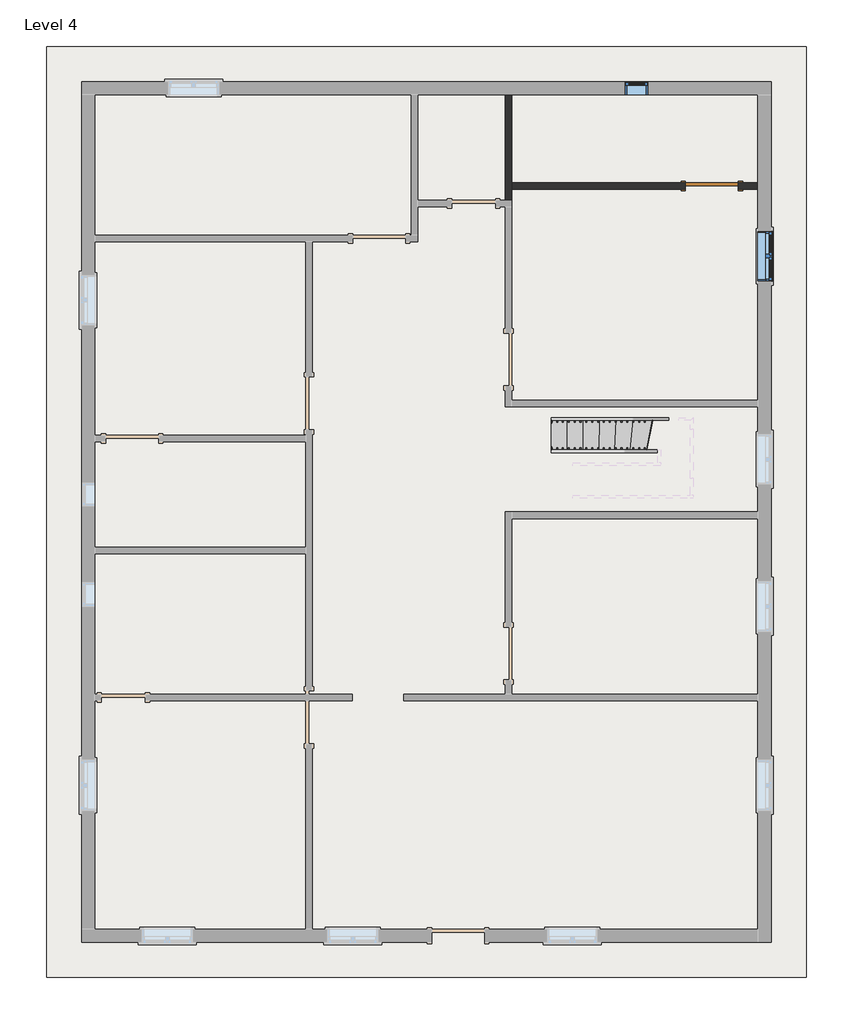
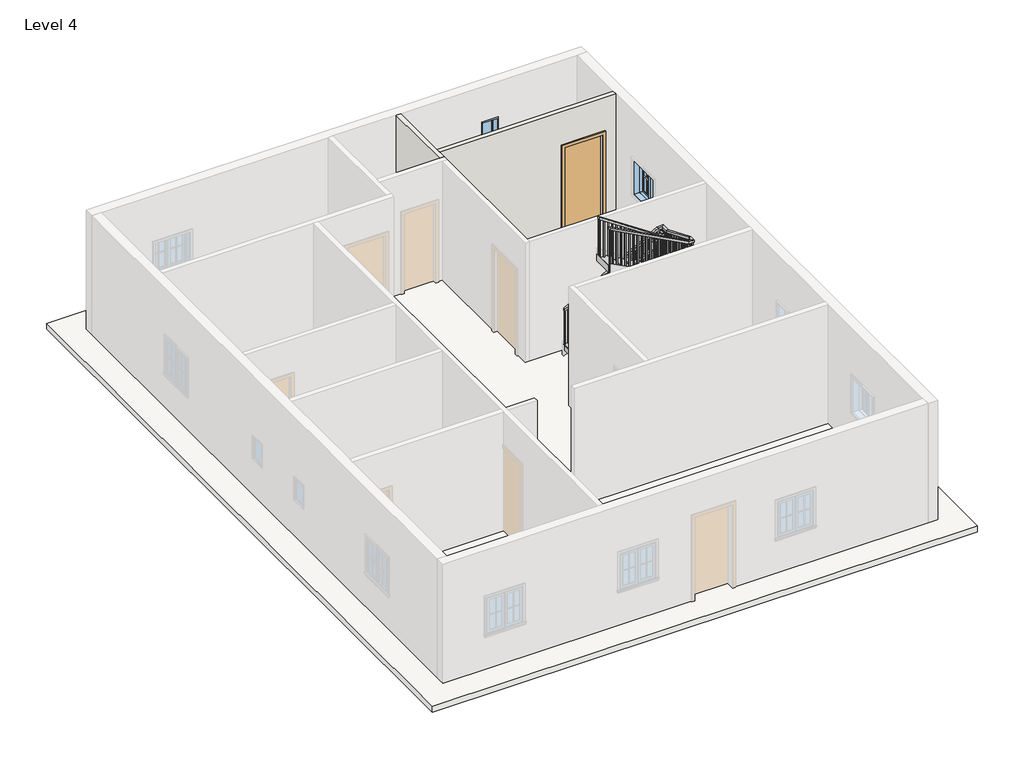
# One storey, part 2 of 3: 2 railings, 2 walls, 2 windows, 1 door, 1 roof, 1 stair flight.
"""IFC4 building model written with IfcOpenShell, lengths in millimetres."""

from ifc_helpers import new_model, si_unit, frame, origin, place, context, project, spatial, polyline, outline, extrude, faceted_brep, transform, mapped, element, save
from components import door_e5f9f3c4, stair_flight_0d5ba797, window_373d1f99, window_339605e1

model = new_model("IFC4")

# Units and contexts
model_context = context("Model", 3, world=origin())
ifc_project = project(units=[si_unit("LENGTHUNIT", "METRE", prefix="MILLI")], contexts=[model_context])

# Site, building, storey
site = spatial("IfcSite", under=ifc_project)
building = spatial("IfcBuilding", under=site)
storey = spatial("IfcBuildingStorey", under=building, Name="Level 4", Elevation=6400.8)

# Door
placement = place(None, origin())
door_shape = door_e5f9f3c4(model_context)
element("IfcDoor", 1, ObjectType="Single-Flush : 36\" x 84\"", at=placement, inside=storey, context=model_context, shape_type="MappedRepresentation", body=[
    mapped(door_shape, transform((3624.6756993, 7272.227558, 6400.8), x_axis=(1.0, 0.0, 0.0), y_axis=(0.0, 1.0, 0.0), z_axis=(0.0, 0.0, 1.0))),
])

# Railings
element("IfcRailing", 2, ObjectType="Handrail - Rectangular", at=placement, inside=storey, context=model_context, shape_type="SolidModel", body=[
    faceted_brep([(838.4202681, 2744.677558, 7653.8666667), (838.4202681, 2744.677558, 7593.5442501), (838.4202681, 2693.877558, 7593.5442501), (838.4202681, 2693.877558, 7653.8666667), (2663.2073911, 2744.677558, 8822.3510761), (2714.0073911, 2744.677558, 8794.5579377), (2714.0073911, 2693.877558, 8794.5579377), (2663.2073911, 2693.877558, 8822.3510761), (2663.2073911, 2744.677558, 9034.6070819), (2714.0073911, 2744.677558, 8983.8070819), (2714.0073911, 2693.877558, 8983.8070819), (2663.2073911, 2693.877558, 9034.6070819), (2790.2073911, 2744.677558, 9034.6070819), (2790.2073911, 2744.677558, 8983.8070819), (2739.4073911, 2693.877558, 8983.8070819), (2739.4073911, 2693.877558, 9034.6070819), (2790.2073911, 2617.677558, 9034.6070819), (2790.2073911, 2595.5706127, 8983.8070819), (2739.4073911, 2595.5706127, 8983.8070819), (2739.4073911, 2617.677558, 9034.6070819), (2790.2073911, 2490.677558, 9170.9650362), (2790.2073911, 2439.877558, 9150.9723294), (2739.4073911, 2439.877558, 9150.9723294), (2739.4073911, 2490.677558, 9170.9650362), (2790.2073911, 2490.677558, 9386.5137911), (2790.2073911, 2439.877558, 9335.7137911), (2739.4073911, 2439.877558, 9335.7137911), (2739.4073911, 2490.677558, 9386.5137911), (2790.2073911, 2363.677558, 9386.5137911), (2790.2073911, 2363.677558, 9335.7137911), (2739.4073911, 2414.477558, 9335.7137911), (2739.4073911, 2414.477558, 9386.5137911), (2663.2073911, 2363.677558, 9386.5137911), (2647.7076469, 2363.677558, 9335.7137911), (2647.7076469, 2414.477558, 9335.7137911), (2663.2073911, 2414.477558, 9386.5137911), (1211.6756993, 2363.677558, 10363.2), (1211.6756993, 2414.477558, 10363.2), (1211.6756993, 2414.477558, 10301.9707504), (1211.6756993, 2363.677558, 10301.9707504)], [[[0, 1, 2, 3]], [[1, 0, 4, 5]], [[2, 1, 5, 6]], [[3, 2, 6, 7]], [[0, 3, 7, 4]], [[5, 4, 8, 9]], [[6, 5, 9, 10]], [[7, 6, 10, 11]], [[4, 7, 11, 8]], [[9, 8, 12, 13]], [[10, 9, 13, 14]], [[11, 10, 14, 15]], [[8, 11, 15, 12]], [[13, 12, 16, 17]], [[14, 13, 17, 18]], [[15, 14, 18, 19]], [[12, 15, 19, 16]], [[17, 16, 20, 21]], [[18, 17, 21, 22]], [[19, 18, 22, 23]], [[16, 19, 23, 20]], [[21, 20, 24, 25]], [[22, 21, 25, 26]], [[23, 22, 26, 27]], [[20, 23, 27, 24]], [[25, 24, 28, 29]], [[26, 25, 29, 30]], [[27, 26, 30, 31]], [[24, 27, 31, 28]], [[29, 28, 32, 33]], [[30, 29, 33, 34]], [[31, 30, 34, 35]], [[28, 31, 35, 32]], [[36, 37, 38, 39]], [[33, 32, 36, 39]], [[34, 33, 39, 38]], [[35, 34, 38, 37]], [[32, 35, 37, 36]]]),
    extrude(outline(polyline([(10275.9599798, 1250.3323911), (10288.7780756, 1231.2823911), (9279.4666667, 1231.2823911), (9279.4666667, 1250.3323911), (10275.9599798, 1250.3323911)])), frame((0.0, 2379.552558, 0.0), z_axis=(0.0, 1.0, 0.0), x_axis=(0.0, 0.0, 1.0)), (0.0, 0.0, 1.0), 19.05),
    extrude(outline(polyline([(10207.5968022, 1351.9323911), (10220.414898, 1332.8823911), (9279.4666667, 1332.8823911), (9279.4666667, 1351.9323911), (10207.5968022, 1351.9323911)])), frame((0.0, 2379.552558, 0.0), z_axis=(0.0, 1.0, 0.0), x_axis=(0.0, 0.0, 1.0)), (0.0, 0.0, 1.0), 19.05),
    extrude(outline(polyline([(10139.2336246, 1453.5323911), (10152.0517204, 1434.4823911), (9279.4666667, 1434.4823911), (9279.4666667, 1453.5323911), (10139.2336246, 1453.5323911)])), frame((0.0, 2379.552558, 0.0), z_axis=(0.0, 1.0, 0.0), x_axis=(0.0, 0.0, 1.0)), (0.0, 0.0, 1.0), 19.05),
    extrude(outline(polyline([(10070.870447, 1555.1323911), (10083.6885428, 1536.0823911), (9110.1333333, 1536.0823911), (9110.1333333, 1555.1323911), (10070.870447, 1555.1323911)])), frame((0.0, 2379.552558, 0.0), z_axis=(0.0, 1.0, 0.0), x_axis=(0.0, 0.0, 1.0)), (0.0, 0.0, 1.0), 19.05),
    extrude(outline(polyline([(10002.5072694, 1656.7323911), (10015.3253652, 1637.6823911), (9110.1333333, 1637.6823911), (9110.1333333, 1656.7323911), (10002.5072694, 1656.7323911)])), frame((0.0, 2379.552558, 0.0), z_axis=(0.0, 1.0, 0.0), x_axis=(0.0, 0.0, 1.0)), (0.0, 0.0, 1.0), 19.05),
    extrude(outline(polyline([(9934.1440918, 1758.3323911), (9946.9621876, 1739.2823911), (9110.1333333, 1739.2823911), (9110.1333333, 1758.3323911), (9934.1440918, 1758.3323911)])), frame((0.0, 2379.552558, 0.0), z_axis=(0.0, 1.0, 0.0), x_axis=(0.0, 0.0, 1.0)), (0.0, 0.0, 1.0), 19.05),
    extrude(outline(polyline([(9865.7809143, 1859.9323911), (9878.5990101, 1840.8823911), (8940.8, 1840.8823911), (8940.8, 1859.9323911), (9865.7809143, 1859.9323911)])), frame((0.0, 2379.552558, 0.0), z_axis=(0.0, 1.0, 0.0), x_axis=(0.0, 0.0, 1.0)), (0.0, 0.0, 1.0), 19.05),
    extrude(outline(polyline([(9797.4177367, 1961.5323911), (9810.2358325, 1942.4823911), (8940.8, 1942.4823911), (8940.8, 1961.5323911), (9797.4177367, 1961.5323911)])), frame((0.0, 2379.552558, 0.0), z_axis=(0.0, 1.0, 0.0), x_axis=(0.0, 0.0, 1.0)), (0.0, 0.0, 1.0), 19.05),
    extrude(outline(polyline([(9729.0545591, 2063.1323911), (9741.8726549, 2044.0823911), (8771.4666667, 2044.0823911), (8771.4666667, 2063.1323911), (9729.0545591, 2063.1323911)])), frame((0.0, 2379.552558, 0.0), z_axis=(0.0, 1.0, 0.0), x_axis=(0.0, 0.0, 1.0)), (0.0, 0.0, 1.0), 19.05),
    extrude(outline(polyline([(9660.6913815, 2164.7323911), (9673.5094773, 2145.6823911), (8771.4666667, 2145.6823911), (8771.4666667, 2164.7323911), (9660.6913815, 2164.7323911)])), frame((0.0, 2379.552558, 0.0), z_axis=(0.0, 1.0, 0.0), x_axis=(0.0, 0.0, 1.0)), (0.0, 0.0, 1.0), 19.05),
    extrude(outline(polyline([(9592.3282039, 2266.3323911), (9605.1462997, 2247.2823911), (8771.4666667, 2247.2823911), (8771.4666667, 2266.3323911), (9592.3282039, 2266.3323911)])), frame((0.0, 2379.552558, 0.0), z_axis=(0.0, 1.0, 0.0), x_axis=(0.0, 0.0, 1.0)), (0.0, 0.0, 1.0), 19.05),
    extrude(outline(polyline([(9523.9650263, 2367.9323911), (9536.7831221, 2348.8823911), (8602.1333333, 2348.8823911), (8602.1333333, 2367.9323911), (9523.9650263, 2367.9323911)])), frame((0.0, 2379.552558, 0.0), z_axis=(0.0, 1.0, 0.0), x_axis=(0.0, 0.0, 1.0)), (0.0, 0.0, 1.0), 19.05),
    extrude(outline(polyline([(9455.6018487, 2469.5323911), (9468.4199445, 2450.4823911), (8602.1333333, 2450.4823911), (8602.1333333, 2469.5323911), (9455.6018487, 2469.5323911)])), frame((0.0, 2379.552558, 0.0), z_axis=(0.0, 1.0, 0.0), x_axis=(0.0, 0.0, 1.0)), (0.0, 0.0, 1.0), 19.05),
    extrude(outline(polyline([(9387.2386712, 2571.1323911), (9400.056767, 2552.0823911), (8432.8, 2552.0823911), (8432.8, 2571.1323911), (9387.2386712, 2571.1323911)])), frame((0.0, 2379.552558, 0.0), z_axis=(0.0, 1.0, 0.0), x_axis=(0.0, 0.0, 1.0)), (0.0, 0.0, 1.0), 19.05),
    extrude(outline(polyline([(9318.8754936, 2672.7323911), (9331.6935894, 2653.6823911), (8432.8, 2653.6823911), (8432.8, 2672.7323911), (9318.8754936, 2672.7323911)])), frame((0.0, 2379.552558, 0.0), z_axis=(0.0, 1.0, 0.0), x_axis=(0.0, 0.0, 1.0)), (0.0, 0.0, 1.0), 19.05),
    extrude(outline(polyline([(2755.2823911, 2424.002558), (2774.3323911, 2424.002558), (2774.3323911, 2404.952558), (2755.2823911, 2404.952558), (2755.2823911, 2424.002558)])), frame((0.0, 0.0, 8263.4666667), z_axis=(0.0, 0.0, 1.0), x_axis=(1.0, 0.0, 0.0)), (0.0, 0.0, 1.0), 1072.2471245),
    extrude(outline(polyline([(2506.552558, 9079.3844034), (2525.602558, 9058.9307103), (2525.602558, 8094.1333333), (2506.552558, 8094.1333333), (2506.552558, 9079.3844034)])), frame((2755.2823911, 0.0, 0.0), z_axis=(1.0, 0.0, 0.0), x_axis=(0.0, 1.0, 0.0)), (0.0, 0.0, 1.0), 19.05),
    extrude(outline(polyline([(2608.152558, 8970.29804), (2627.202558, 8949.8443468), (2627.202558, 8094.1333333), (2608.152558, 8094.1333333), (2608.152558, 8970.29804)])), frame((2755.2823911, 0.0, 0.0), z_axis=(1.0, 0.0, 0.0), x_axis=(0.0, 1.0, 0.0)), (0.0, 0.0, 1.0), 19.05),
    extrude(outline(polyline([(2657.6952681, 2709.752558), (2657.6952681, 2728.802558), (2676.7452681, 2728.802558), (2676.7452681, 2709.752558), (2657.6952681, 2709.752558)])), frame((0.0, 0.0, 7755.4666667), z_axis=(0.0, 0.0, 1.0), x_axis=(1.0, 0.0, 0.0)), (0.0, 0.0, 1.0), 1228.3404152),
    extrude(outline(polyline([(8705.6389489, 2575.1452681), (8693.4404695, 2556.0952681), (7755.4666667, 2556.0952681), (7755.4666667, 2575.1452681), (8705.6389489, 2575.1452681)])), frame((0.0, 2709.752558, 0.0), z_axis=(0.0, 1.0, 0.0), x_axis=(0.0, 0.0, 1.0)), (0.0, 0.0, 1.0), 19.05),
    extrude(outline(polyline([(8640.5803925, 2473.5452681), (8628.3819131, 2454.4952681), (7586.1333333, 2454.4952681), (7586.1333333, 2473.5452681), (8640.5803925, 2473.5452681)])), frame((0.0, 2709.752558, 0.0), z_axis=(0.0, 1.0, 0.0), x_axis=(0.0, 0.0, 1.0)), (0.0, 0.0, 1.0), 19.05),
    extrude(outline(polyline([(8575.521836, 2371.9452681), (8563.3233567, 2352.8952681), (7586.1333333, 2352.8952681), (7586.1333333, 2371.9452681), (8575.521836, 2371.9452681)])), frame((0.0, 2709.752558, 0.0), z_axis=(0.0, 1.0, 0.0), x_axis=(0.0, 0.0, 1.0)), (0.0, 0.0, 1.0), 19.05),
    extrude(outline(polyline([(8510.4632796, 2270.3452681), (8498.2648003, 2251.2952681), (7586.1333333, 2251.2952681), (7586.1333333, 2270.3452681), (8510.4632796, 2270.3452681)])), frame((0.0, 2709.752558, 0.0), z_axis=(0.0, 1.0, 0.0), x_axis=(0.0, 0.0, 1.0)), (0.0, 0.0, 1.0), 19.05),
    extrude(outline(polyline([(8445.4047232, 2168.7452681), (8433.2062439, 2149.6952681), (7416.8, 2149.6952681), (7416.8, 2168.7452681), (8445.4047232, 2168.7452681)])), frame((0.0, 2709.752558, 0.0), z_axis=(0.0, 1.0, 0.0), x_axis=(0.0, 0.0, 1.0)), (0.0, 0.0, 1.0), 19.05),
    extrude(outline(polyline([(8380.3461668, 2067.1452681), (8368.1476875, 2048.0952681), (7416.8, 2048.0952681), (7416.8, 2067.1452681), (8380.3461668, 2067.1452681)])), frame((0.0, 2709.752558, 0.0), z_axis=(0.0, 1.0, 0.0), x_axis=(0.0, 0.0, 1.0)), (0.0, 0.0, 1.0), 19.05),
    extrude(outline(polyline([(8315.2876104, 1965.5452681), (8303.089131, 1946.4952681), (7416.8, 1946.4952681), (7416.8, 1965.5452681), (8315.2876104, 1965.5452681)])), frame((0.0, 2709.752558, 0.0), z_axis=(0.0, 1.0, 0.0), x_axis=(0.0, 0.0, 1.0)), (0.0, 0.0, 1.0), 19.05),
    extrude(outline(polyline([(8250.2290539, 1863.9452681), (8238.0305746, 1844.8952681), (7247.4666667, 1844.8952681), (7247.4666667, 1863.9452681), (8250.2290539, 1863.9452681)])), frame((0.0, 2709.752558, 0.0), z_axis=(0.0, 1.0, 0.0), x_axis=(0.0, 0.0, 1.0)), (0.0, 0.0, 1.0), 19.05),
    extrude(outline(polyline([(8185.1704975, 1762.3452681), (8172.9720182, 1743.2952681), (7247.4666667, 1743.2952681), (7247.4666667, 1762.3452681), (8185.1704975, 1762.3452681)])), frame((0.0, 2709.752558, 0.0), z_axis=(0.0, 1.0, 0.0), x_axis=(0.0, 0.0, 1.0)), (0.0, 0.0, 1.0), 19.05),
    extrude(outline(polyline([(8120.1119411, 1660.7452681), (8107.9134618, 1641.6952681), (7078.1333333, 1641.6952681), (7078.1333333, 1660.7452681), (8120.1119411, 1660.7452681)])), frame((0.0, 2709.752558, 0.0), z_axis=(0.0, 1.0, 0.0), x_axis=(0.0, 0.0, 1.0)), (0.0, 0.0, 1.0), 19.05),
    extrude(outline(polyline([(8055.0533847, 1559.1452681), (8042.8549054, 1540.0952681), (7078.1333333, 1540.0952681), (7078.1333333, 1559.1452681), (8055.0533847, 1559.1452681)])), frame((0.0, 2709.752558, 0.0), z_axis=(0.0, 1.0, 0.0), x_axis=(0.0, 0.0, 1.0)), (0.0, 0.0, 1.0), 19.05),
    extrude(outline(polyline([(7989.9948283, 1457.5452681), (7977.7963489, 1438.4952681), (7078.1333333, 1438.4952681), (7078.1333333, 1457.5452681), (7989.9948283, 1457.5452681)])), frame((0.0, 2709.752558, 0.0), z_axis=(0.0, 1.0, 0.0), x_axis=(0.0, 0.0, 1.0)), (0.0, 0.0, 1.0), 19.05),
    extrude(outline(polyline([(7924.9362719, 1355.9452681), (7912.7377925, 1336.8952681), (6908.8, 1336.8952681), (6908.8, 1355.9452681), (7924.9362719, 1355.9452681)])), frame((0.0, 2709.752558, 0.0), z_axis=(0.0, 1.0, 0.0), x_axis=(0.0, 0.0, 1.0)), (0.0, 0.0, 1.0), 19.05),
    extrude(outline(polyline([(7859.8777154, 1254.3452681), (7847.6792361, 1235.2952681), (6908.8, 1235.2952681), (6908.8, 1254.3452681), (7859.8777154, 1254.3452681)])), frame((0.0, 2709.752558, 0.0), z_axis=(0.0, 1.0, 0.0), x_axis=(0.0, 0.0, 1.0)), (0.0, 0.0, 1.0), 19.05),
    extrude(outline(polyline([(7794.819159, 1152.7452681), (7782.6206797, 1133.6952681), (6908.8, 1133.6952681), (6908.8, 1152.7452681), (7794.819159, 1152.7452681)])), frame((0.0, 2709.752558, 0.0), z_axis=(0.0, 1.0, 0.0), x_axis=(0.0, 0.0, 1.0)), (0.0, 0.0, 1.0), 19.05),
    extrude(outline(polyline([(7729.7606026, 1051.1452681), (7717.5621233, 1032.0952681), (6739.4666667, 1032.0952681), (6739.4666667, 1051.1452681), (7729.7606026, 1051.1452681)])), frame((0.0, 2709.752558, 0.0), z_axis=(0.0, 1.0, 0.0), x_axis=(0.0, 0.0, 1.0)), (0.0, 0.0, 1.0), 19.05),
    extrude(outline(polyline([(7664.7020462, 949.5452681), (7652.5035669, 930.4952681), (6739.4666667, 930.4952681), (6739.4666667, 949.5452681), (7664.7020462, 949.5452681)])), frame((0.0, 2709.752558, 0.0), z_axis=(0.0, 1.0, 0.0), x_axis=(0.0, 0.0, 1.0)), (0.0, 0.0, 1.0), 19.05),
    extrude(outline(polyline([(2755.2823911, 2398.602558), (2774.3323911, 2398.602558), (2774.3323911, 2379.552558), (2755.2823911, 2379.552558), (2755.2823911, 2398.602558)])), frame((0.0, 0.0, 8263.4666667), z_axis=(0.0, 0.0, 1.0), x_axis=(1.0, 0.0, 0.0)), (0.0, 0.0, 1.0), 1072.2471245),
    extrude(outline(polyline([(2755.2823911, 2709.752558), (2755.2823911, 2728.802558), (2774.3323911, 2728.802558), (2774.3323911, 2709.752558), (2755.2823911, 2709.752558)])), frame((0.0, 0.0, 7924.8), z_axis=(0.0, 0.0, 1.0), x_axis=(1.0, 0.0, 0.0)), (0.0, 0.0, 1.0), 1059.0070819),
    extrude(outline(polyline([(10289.1526546, 1230.7256993), (10301.9707504, 1211.6756993), (9279.4666667, 1211.6756993), (9279.4666667, 1230.7256993), (10289.1526546, 1230.7256993)])), frame((0.0, 2379.552558, 0.0), z_axis=(0.0, 1.0, 0.0), x_axis=(0.0, 0.0, 1.0)), (0.0, 0.0, 1.0), 19.05),
    extrude(outline(polyline([(7605.7427294, 857.4702681), (7593.5442501, 838.4202681), (6739.4666667, 838.4202681), (6739.4666667, 857.4702681), (7605.7427294, 857.4702681)])), frame((0.0, 2709.752558, 0.0), z_axis=(0.0, 1.0, 0.0), x_axis=(0.0, 0.0, 1.0)), (0.0, 0.0, 1.0), 19.05),
])
element("IfcRailing", 3, ObjectType="Handrail - Rectangular", at=placement, inside=storey, context=model_context, shape_type="SolidModel", body=[
    faceted_brep([(838.4202681, 3202.4524989, 7653.8666667), (838.4202681, 3202.4524989, 7595.2953096), (838.4202681, 3151.6524989, 7595.2953096), (838.4202681, 3151.6524989, 7653.8666667), (3089.9785641, 3202.4524989, 8946.0368493), (3103.5198636, 3202.4524989, 8895.2368493), (3103.5198636, 3151.6524989, 8895.2368493), (3089.9785641, 3151.6524989, 8946.0368493), (3247.982332, 3202.4524989, 8946.0368493), (3247.982332, 3202.4524989, 8895.2368493), (3197.182332, 3151.6524989, 8895.2368493), (3197.182332, 3151.6524989, 8946.0368493), (3247.982332, 2995.1725832, 8946.0368493), (3247.982332, 2984.9732412, 8895.2368493), (3197.182332, 2984.9732412, 8895.2368493), (3197.182332, 2995.1725832, 8946.0368493), (3247.982332, 2050.6126885, 9341.2552365), (3247.982332, 2040.4133465, 9290.4552365), (3197.182332, 2040.4133465, 9290.4552365), (3197.182332, 2050.6126885, 9341.2552365), (3247.982332, 1905.9026171, 9341.2552365), (3247.982332, 1905.9026171, 9290.4552365), (3197.182332, 1956.7026171, 9290.4552365), (3197.182332, 1956.7026171, 9341.2552365), (3128.9262072, 1905.9026171, 9341.2552365), (3116.2326609, 1905.9026171, 9290.4552365), (3116.2326609, 1956.7026171, 9290.4552365), (3128.9262072, 1956.7026171, 9341.2552365), (1211.6756993, 1905.9026171, 10363.2), (1211.6756993, 1956.7026171, 10363.2), (1211.6756993, 1956.7026171, 10305.6340072), (1211.6756993, 1905.9026171, 10305.6340072)], [[[0, 1, 2, 3]], [[1, 0, 4, 5]], [[2, 1, 5, 6]], [[3, 2, 6, 7]], [[0, 3, 7, 4]], [[5, 4, 8, 9]], [[6, 5, 9, 10]], [[7, 6, 10, 11]], [[4, 7, 11, 8]], [[9, 8, 12, 13]], [[10, 9, 13, 14]], [[11, 10, 14, 15]], [[8, 11, 15, 12]], [[13, 12, 16, 17]], [[14, 13, 17, 18]], [[15, 14, 18, 19]], [[12, 15, 19, 16]], [[17, 16, 20, 21]], [[18, 17, 21, 22]], [[19, 18, 22, 23]], [[16, 19, 23, 20]], [[21, 20, 24, 25]], [[22, 21, 25, 26]], [[23, 22, 26, 27]], [[20, 23, 27, 24]], [[28, 29, 30, 31]], [[25, 24, 28, 31]], [[26, 25, 31, 30]], [[27, 26, 30, 29]], [[24, 27, 29, 28]]]),
    extrude(outline(polyline([(10267.7989368, 1282.657332), (9279.4666667, 1282.657332), (9279.4666667, 1301.707332), (10257.6447876, 1301.707332), (10267.7989368, 1282.657332)])), frame((0.0, 1921.7776171, 0.0), z_axis=(0.0, 1.0, 0.0), x_axis=(0.0, 0.0, 1.0)), (0.0, 0.0, 1.0), 19.05),
    extrude(outline(polyline([(10213.6434743, 1384.257332), (9279.4666667, 1384.257332), (9279.4666667, 1403.307332), (10203.4893251, 1403.307332), (10213.6434743, 1384.257332)])), frame((0.0, 1921.7776171, 0.0), z_axis=(0.0, 1.0, 0.0), x_axis=(0.0, 0.0, 1.0)), (0.0, 0.0, 1.0), 19.05),
    extrude(outline(polyline([(10159.4880118, 1485.857332), (9110.1333333, 1485.857332), (9110.1333333, 1504.907332), (10149.3338626, 1504.907332), (10159.4880118, 1485.857332)])), frame((0.0, 1921.7776171, 0.0), z_axis=(0.0, 1.0, 0.0), x_axis=(0.0, 0.0, 1.0)), (0.0, 0.0, 1.0), 19.05),
    extrude(outline(polyline([(10105.3325493, 1587.457332), (9110.1333333, 1587.457332), (9110.1333333, 1606.507332), (10095.1784001, 1606.507332), (10105.3325493, 1587.457332)])), frame((0.0, 1921.7776171, 0.0), z_axis=(0.0, 1.0, 0.0), x_axis=(0.0, 0.0, 1.0)), (0.0, 0.0, 1.0), 19.05),
    extrude(outline(polyline([(10051.1770868, 1689.057332), (9110.1333333, 1689.057332), (9110.1333333, 1708.107332), (10041.0229376, 1708.107332), (10051.1770868, 1689.057332)])), frame((0.0, 1921.7776171, 0.0), z_axis=(0.0, 1.0, 0.0), x_axis=(0.0, 0.0, 1.0)), (0.0, 0.0, 1.0), 19.05),
    extrude(outline(polyline([(9997.0216243, 1790.657332), (8940.8, 1790.657332), (8940.8, 1809.707332), (9986.8674751, 1809.707332), (9997.0216243, 1790.657332)])), frame((0.0, 1921.7776171, 0.0), z_axis=(0.0, 1.0, 0.0), x_axis=(0.0, 0.0, 1.0)), (0.0, 0.0, 1.0), 19.05),
    extrude(outline(polyline([(9942.8661618, 1892.257332), (8940.8, 1892.257332), (8940.8, 1911.307332), (9932.7120126, 1911.307332), (9942.8661618, 1892.257332)])), frame((0.0, 1921.7776171, 0.0), z_axis=(0.0, 1.0, 0.0), x_axis=(0.0, 0.0, 1.0)), (0.0, 0.0, 1.0), 19.05),
    extrude(outline(polyline([(9888.7106993, 1993.857332), (8940.8, 1993.857332), (8940.8, 2012.907332), (9878.5565501, 2012.907332), (9888.7106993, 1993.857332)])), frame((0.0, 1921.7776171, 0.0), z_axis=(0.0, 1.0, 0.0), x_axis=(0.0, 0.0, 1.0)), (0.0, 0.0, 1.0), 19.05),
    extrude(outline(polyline([(9834.5552369, 2095.457332), (8771.4666667, 2095.457332), (8771.4666667, 2114.507332), (9824.4010876, 2114.507332), (9834.5552369, 2095.457332)])), frame((0.0, 1921.7776171, 0.0), z_axis=(0.0, 1.0, 0.0), x_axis=(0.0, 0.0, 1.0)), (0.0, 0.0, 1.0), 19.05),
    extrude(outline(polyline([(9780.3997744, 2197.057332), (8771.4666667, 2197.057332), (8771.4666667, 2216.107332), (9770.2456251, 2216.107332), (9780.3997744, 2197.057332)])), frame((0.0, 1921.7776171, 0.0), z_axis=(0.0, 1.0, 0.0), x_axis=(0.0, 0.0, 1.0)), (0.0, 0.0, 1.0), 19.05),
    extrude(outline(polyline([(9726.2443119, 2298.657332), (8771.4666667, 2298.657332), (8771.4666667, 2317.707332), (9716.0901626, 2317.707332), (9726.2443119, 2298.657332)])), frame((0.0, 1921.7776171, 0.0), z_axis=(0.0, 1.0, 0.0), x_axis=(0.0, 0.0, 1.0)), (0.0, 0.0, 1.0), 19.05),
    extrude(outline(polyline([(9672.0888494, 2400.257332), (8602.1333333, 2400.257332), (8602.1333333, 2419.307332), (9661.9347002, 2419.307332), (9672.0888494, 2400.257332)])), frame((0.0, 1921.7776171, 0.0), z_axis=(0.0, 1.0, 0.0), x_axis=(0.0, 0.0, 1.0)), (0.0, 0.0, 1.0), 19.05),
    extrude(outline(polyline([(9617.9333869, 2501.857332), (8602.1333333, 2501.857332), (8602.1333333, 2520.907332), (9607.7792377, 2520.907332), (9617.9333869, 2501.857332)])), frame((0.0, 1921.7776171, 0.0), z_axis=(0.0, 1.0, 0.0), x_axis=(0.0, 0.0, 1.0)), (0.0, 0.0, 1.0), 19.05),
    extrude(outline(polyline([(9563.7779244, 2603.457332), (8602.1333333, 2603.457332), (8602.1333333, 2622.507332), (9553.6237752, 2622.507332), (9563.7779244, 2603.457332)])), frame((0.0, 1921.7776171, 0.0), z_axis=(0.0, 1.0, 0.0), x_axis=(0.0, 0.0, 1.0)), (0.0, 0.0, 1.0), 19.05),
    extrude(outline(polyline([(9509.6224619, 2705.057332), (8432.8, 2705.057332), (8432.8, 2724.107332), (9499.4683127, 2724.107332), (9509.6224619, 2705.057332)])), frame((0.0, 1921.7776171, 0.0), z_axis=(0.0, 1.0, 0.0), x_axis=(0.0, 0.0, 1.0)), (0.0, 0.0, 1.0), 19.05),
    extrude(outline(polyline([(9455.4669994, 2806.657332), (8432.8, 2806.657332), (8432.8, 2825.707332), (9445.3128502, 2825.707332), (9455.4669994, 2806.657332)])), frame((0.0, 1921.7776171, 0.0), z_axis=(0.0, 1.0, 0.0), x_axis=(0.0, 0.0, 1.0)), (0.0, 0.0, 1.0), 19.05),
    extrude(outline(polyline([(9401.3115369, 2908.257332), (8432.8, 2908.257332), (8432.8, 2927.307332), (9391.1573877, 2927.307332), (9401.3115369, 2908.257332)])), frame((0.0, 1921.7776171, 0.0), z_axis=(0.0, 1.0, 0.0), x_axis=(0.0, 0.0, 1.0)), (0.0, 0.0, 1.0), 19.05),
    extrude(outline(polyline([(9347.1560744, 3009.857332), (8432.8, 3009.857332), (8432.8, 3028.907332), (9337.0019252, 3028.907332), (9347.1560744, 3009.857332)])), frame((0.0, 1921.7776171, 0.0), z_axis=(0.0, 1.0, 0.0), x_axis=(0.0, 0.0, 1.0)), (0.0, 0.0, 1.0), 19.05),
    extrude(outline(polyline([(9293.0006119, 3111.457332), (8263.4666667, 3111.457332), (8263.4666667, 3130.507332), (9282.8464627, 3130.507332), (9293.0006119, 3111.457332)])), frame((0.0, 1921.7776171, 0.0), z_axis=(0.0, 1.0, 0.0), x_axis=(0.0, 0.0, 1.0)), (0.0, 0.0, 1.0), 19.05),
    extrude(outline(polyline([(3232.107332, 1967.3774989), (3232.107332, 1948.3274989), (3213.057332, 1948.3274989), (3213.057332, 1967.3774989), (3232.107332, 1967.3774989)])), frame((0.0, 0.0, 8263.4666667), z_axis=(0.0, 0.0, 1.0), x_axis=(1.0, 0.0, 0.0)), (0.0, 0.0, 1.0), 1026.9885698),
    extrude(outline(polyline([(2068.9774989, 9278.5035558), (2068.9774989, 8263.4666667), (2049.9274989, 8263.4666667), (2049.9274989, 9286.4743688), (2068.9774989, 9278.5035558)])), frame((3213.057332, 0.0, 0.0), z_axis=(1.0, 0.0, 0.0), x_axis=(0.0, 1.0, 0.0)), (0.0, 0.0, 1.0), 19.05),
    extrude(outline(polyline([(2170.5774989, 9235.9925532), (2170.5774989, 8263.4666667), (2151.5274989, 8263.4666667), (2151.5274989, 9243.9633662), (2170.5774989, 9235.9925532)])), frame((3213.057332, 0.0, 0.0), z_axis=(1.0, 0.0, 0.0), x_axis=(0.0, 1.0, 0.0)), (0.0, 0.0, 1.0), 19.05),
    extrude(outline(polyline([(2272.1774989, 9193.4815506), (2272.1774989, 8263.4666667), (2253.1274989, 8263.4666667), (2253.1274989, 9201.4523636), (2272.1774989, 9193.4815506)])), frame((3213.057332, 0.0, 0.0), z_axis=(1.0, 0.0, 0.0), x_axis=(0.0, 1.0, 0.0)), (0.0, 0.0, 1.0), 19.05),
    extrude(outline(polyline([(2373.7774989, 9150.970548), (2373.7774989, 8263.4666667), (2354.7274989, 8263.4666667), (2354.7274989, 9158.941361), (2373.7774989, 9150.970548)])), frame((3213.057332, 0.0, 0.0), z_axis=(1.0, 0.0, 0.0), x_axis=(0.0, 1.0, 0.0)), (0.0, 0.0, 1.0), 19.05),
    extrude(outline(polyline([(2475.3774989, 9108.4595454), (2475.3774989, 8094.1333333), (2456.3274989, 8094.1333333), (2456.3274989, 9116.4303584), (2475.3774989, 9108.4595454)])), frame((3213.057332, 0.0, 0.0), z_axis=(1.0, 0.0, 0.0), x_axis=(0.0, 1.0, 0.0)), (0.0, 0.0, 1.0), 19.05),
    extrude(outline(polyline([(2576.9774989, 9065.9485428), (2576.9774989, 8094.1333333), (2557.9274989, 8094.1333333), (2557.9274989, 9073.9193558), (2576.9774989, 9065.9485428)])), frame((3213.057332, 0.0, 0.0), z_axis=(1.0, 0.0, 0.0), x_axis=(0.0, 1.0, 0.0)), (0.0, 0.0, 1.0), 19.05),
    extrude(outline(polyline([(2678.5774989, 9023.4375402), (2678.5774989, 8094.1333333), (2659.5274989, 8094.1333333), (2659.5274989, 9031.4083532), (2678.5774989, 9023.4375402)])), frame((3213.057332, 0.0, 0.0), z_axis=(1.0, 0.0, 0.0), x_axis=(0.0, 1.0, 0.0)), (0.0, 0.0, 1.0), 19.05),
    extrude(outline(polyline([(2780.1774989, 8980.9265376), (2780.1774989, 8094.1333333), (2761.1274989, 8094.1333333), (2761.1274989, 8988.8973506), (2780.1774989, 8980.9265376)])), frame((3213.057332, 0.0, 0.0), z_axis=(1.0, 0.0, 0.0), x_axis=(0.0, 1.0, 0.0)), (0.0, 0.0, 1.0), 19.05),
    extrude(outline(polyline([(2881.7774989, 8938.415535), (2881.7774989, 7924.8), (2862.7274989, 7924.8), (2862.7274989, 8946.386348), (2881.7774989, 8938.415535)])), frame((3213.057332, 0.0, 0.0), z_axis=(1.0, 0.0, 0.0), x_axis=(0.0, 1.0, 0.0)), (0.0, 0.0, 1.0), 19.05),
    extrude(outline(polyline([(2983.3774989, 8895.9045324), (2983.3774989, 7924.8), (2964.3274989, 7924.8), (2964.3274989, 8903.8753454), (2983.3774989, 8895.9045324)])), frame((3213.057332, 0.0, 0.0), z_axis=(1.0, 0.0, 0.0), x_axis=(0.0, 1.0, 0.0)), (0.0, 0.0, 1.0), 19.05),
    extrude(outline(polyline([(3232.107332, 3084.9774989), (3232.107332, 3065.9274989), (3213.057332, 3065.9274989), (3213.057332, 3084.9774989), (3232.107332, 3084.9774989)])), frame((0.0, 0.0, 7924.8), z_axis=(0.0, 0.0, 1.0), x_axis=(1.0, 0.0, 0.0)), (0.0, 0.0, 1.0), 970.4368493),
    extrude(outline(polyline([(3165.6952681, 3186.5774989), (3184.7452681, 3186.5774989), (3184.7452681, 3167.5274989), (3165.6952681, 3167.5274989), (3165.6952681, 3186.5774989)])), frame((0.0, 0.0, 7924.8), z_axis=(0.0, 0.0, 1.0), x_axis=(1.0, 0.0, 0.0)), (0.0, 0.0, 1.0), 970.4368493),
    extrude(outline(polyline([(8872.6110585, 3064.0952681), (7924.8, 3064.0952681), (7924.8, 3083.1452681), (8883.543861, 3083.1452681), (8872.6110585, 3064.0952681)])), frame((0.0, 3167.5274989, 0.0), z_axis=(0.0, 1.0, 0.0), x_axis=(0.0, 0.0, 1.0)), (0.0, 0.0, 1.0), 19.05),
    extrude(outline(polyline([(8814.302779, 2962.4952681), (7924.8, 2962.4952681), (7924.8, 2981.5452681), (8825.2355814, 2981.5452681), (8814.302779, 2962.4952681)])), frame((0.0, 3167.5274989, 0.0), z_axis=(0.0, 1.0, 0.0), x_axis=(0.0, 0.0, 1.0)), (0.0, 0.0, 1.0), 19.05),
    extrude(outline(polyline([(8755.9944994, 2860.8952681), (7755.4666667, 2860.8952681), (7755.4666667, 2879.9452681), (8766.9273019, 2879.9452681), (8755.9944994, 2860.8952681)])), frame((0.0, 3167.5274989, 0.0), z_axis=(0.0, 1.0, 0.0), x_axis=(0.0, 0.0, 1.0)), (0.0, 0.0, 1.0), 19.05),
    extrude(outline(polyline([(8697.6862199, 2759.2952681), (7755.4666667, 2759.2952681), (7755.4666667, 2778.3452681), (8708.6190223, 2778.3452681), (8697.6862199, 2759.2952681)])), frame((0.0, 3167.5274989, 0.0), z_axis=(0.0, 1.0, 0.0), x_axis=(0.0, 0.0, 1.0)), (0.0, 0.0, 1.0), 19.05),
    extrude(outline(polyline([(8639.3779403, 2657.6952681), (7755.4666667, 2657.6952681), (7755.4666667, 2676.7452681), (8650.3107428, 2676.7452681), (8639.3779403, 2657.6952681)])), frame((0.0, 3167.5274989, 0.0), z_axis=(0.0, 1.0, 0.0), x_axis=(0.0, 0.0, 1.0)), (0.0, 0.0, 1.0), 19.05),
    extrude(outline(polyline([(8581.0696608, 2556.0952681), (7755.4666667, 2556.0952681), (7755.4666667, 2575.1452681), (8592.0024632, 2575.1452681), (8581.0696608, 2556.0952681)])), frame((0.0, 3167.5274989, 0.0), z_axis=(0.0, 1.0, 0.0), x_axis=(0.0, 0.0, 1.0)), (0.0, 0.0, 1.0), 19.05),
    extrude(outline(polyline([(8522.7613812, 2454.4952681), (7586.1333333, 2454.4952681), (7586.1333333, 2473.5452681), (8533.6941837, 2473.5452681), (8522.7613812, 2454.4952681)])), frame((0.0, 3167.5274989, 0.0), z_axis=(0.0, 1.0, 0.0), x_axis=(0.0, 0.0, 1.0)), (0.0, 0.0, 1.0), 19.05),
    extrude(outline(polyline([(8464.4531017, 2352.8952681), (7586.1333333, 2352.8952681), (7586.1333333, 2371.9452681), (8475.3859041, 2371.9452681), (8464.4531017, 2352.8952681)])), frame((0.0, 3167.5274989, 0.0), z_axis=(0.0, 1.0, 0.0), x_axis=(0.0, 0.0, 1.0)), (0.0, 0.0, 1.0), 19.05),
    extrude(outline(polyline([(8406.1448221, 2251.2952681), (7586.1333333, 2251.2952681), (7586.1333333, 2270.3452681), (8417.0776245, 2270.3452681), (8406.1448221, 2251.2952681)])), frame((0.0, 3167.5274989, 0.0), z_axis=(0.0, 1.0, 0.0), x_axis=(0.0, 0.0, 1.0)), (0.0, 0.0, 1.0), 19.05),
    extrude(outline(polyline([(8347.8365426, 2149.6952681), (7416.8, 2149.6952681), (7416.8, 2168.7452681), (8358.769345, 2168.7452681), (8347.8365426, 2149.6952681)])), frame((0.0, 3167.5274989, 0.0), z_axis=(0.0, 1.0, 0.0), x_axis=(0.0, 0.0, 1.0)), (0.0, 0.0, 1.0), 19.05),
    extrude(outline(polyline([(8289.528263, 2048.0952681), (7416.8, 2048.0952681), (7416.8, 2067.1452681), (8300.4610654, 2067.1452681), (8289.528263, 2048.0952681)])), frame((0.0, 3167.5274989, 0.0), z_axis=(0.0, 1.0, 0.0), x_axis=(0.0, 0.0, 1.0)), (0.0, 0.0, 1.0), 19.05),
    extrude(outline(polyline([(8231.2199835, 1946.4952681), (7247.4666667, 1946.4952681), (7247.4666667, 1965.5452681), (8242.1527859, 1965.5452681), (8231.2199835, 1946.4952681)])), frame((0.0, 3167.5274989, 0.0), z_axis=(0.0, 1.0, 0.0), x_axis=(0.0, 0.0, 1.0)), (0.0, 0.0, 1.0), 19.05),
    extrude(outline(polyline([(8172.9117039, 1844.8952681), (7247.4666667, 1844.8952681), (7247.4666667, 1863.9452681), (8183.8445063, 1863.9452681), (8172.9117039, 1844.8952681)])), frame((0.0, 3167.5274989, 0.0), z_axis=(0.0, 1.0, 0.0), x_axis=(0.0, 0.0, 1.0)), (0.0, 0.0, 1.0), 19.05),
    extrude(outline(polyline([(8114.6034244, 1743.2952681), (7247.4666667, 1743.2952681), (7247.4666667, 1762.3452681), (8125.5362268, 1762.3452681), (8114.6034244, 1743.2952681)])), frame((0.0, 3167.5274989, 0.0), z_axis=(0.0, 1.0, 0.0), x_axis=(0.0, 0.0, 1.0)), (0.0, 0.0, 1.0), 19.05),
    extrude(outline(polyline([(8056.2951448, 1641.6952681), (7078.1333333, 1641.6952681), (7078.1333333, 1660.7452681), (8067.2279472, 1660.7452681), (8056.2951448, 1641.6952681)])), frame((0.0, 3167.5274989, 0.0), z_axis=(0.0, 1.0, 0.0), x_axis=(0.0, 0.0, 1.0)), (0.0, 0.0, 1.0), 19.05),
    extrude(outline(polyline([(7997.9868653, 1540.0952681), (7078.1333333, 1540.0952681), (7078.1333333, 1559.1452681), (8008.9196677, 1559.1452681), (7997.9868653, 1540.0952681)])), frame((0.0, 3167.5274989, 0.0), z_axis=(0.0, 1.0, 0.0), x_axis=(0.0, 0.0, 1.0)), (0.0, 0.0, 1.0), 19.05),
    extrude(outline(polyline([(7939.6785857, 1438.4952681), (7078.1333333, 1438.4952681), (7078.1333333, 1457.5452681), (7950.6113881, 1457.5452681), (7939.6785857, 1438.4952681)])), frame((0.0, 3167.5274989, 0.0), z_axis=(0.0, 1.0, 0.0), x_axis=(0.0, 0.0, 1.0)), (0.0, 0.0, 1.0), 19.05),
    extrude(outline(polyline([(7881.3703062, 1336.8952681), (6908.8, 1336.8952681), (6908.8, 1355.9452681), (7892.3031086, 1355.9452681), (7881.3703062, 1336.8952681)])), frame((0.0, 3167.5274989, 0.0), z_axis=(0.0, 1.0, 0.0), x_axis=(0.0, 0.0, 1.0)), (0.0, 0.0, 1.0), 19.05),
    extrude(outline(polyline([(7823.0620266, 1235.2952681), (6908.8, 1235.2952681), (6908.8, 1254.3452681), (7833.994829, 1254.3452681), (7823.0620266, 1235.2952681)])), frame((0.0, 3167.5274989, 0.0), z_axis=(0.0, 1.0, 0.0), x_axis=(0.0, 0.0, 1.0)), (0.0, 0.0, 1.0), 19.05),
    extrude(outline(polyline([(7764.628643, 1133.6952681), (6908.8, 1133.6952681), (6908.8, 1152.7452681), (7775.5614454, 1152.7452681), (7764.628643, 1133.6952681)])), frame((0.0, 3167.5274989, 0.0), z_axis=(0.0, 1.0, 0.0), x_axis=(0.0, 0.0, 1.0)), (0.0, 0.0, 1.0), 19.05),
    extrude(outline(polyline([(7706.4454675, 1032.0952681), (6739.4666667, 1032.0952681), (6739.4666667, 1051.1452681), (7717.3782699, 1051.1452681), (7706.4454675, 1032.0952681)])), frame((0.0, 3167.5274989, 0.0), z_axis=(0.0, 1.0, 0.0), x_axis=(0.0, 0.0, 1.0)), (0.0, 0.0, 1.0), 19.05),
    extrude(outline(polyline([(7648.137188, 930.4952681), (6739.4666667, 930.4952681), (6739.4666667, 949.5452681), (7659.0699904, 949.5452681), (7648.137188, 930.4952681)])), frame((0.0, 3167.5274989, 0.0), z_axis=(0.0, 1.0, 0.0), x_axis=(0.0, 0.0, 1.0)), (0.0, 0.0, 1.0), 19.05),
    extrude(outline(polyline([(3232.107332, 1940.8276171), (3232.107332, 1921.7776171), (3213.057332, 1921.7776171), (3213.057332, 1940.8276171), (3232.107332, 1940.8276171)])), frame((0.0, 0.0, 8263.4666667), z_axis=(0.0, 0.0, 1.0), x_axis=(1.0, 0.0, 0.0)), (0.0, 0.0, 1.0), 1026.9885698),
    extrude(outline(polyline([(3213.057332, 3186.5774989), (3232.107332, 3186.5774989), (3232.107332, 3167.5274989), (3213.057332, 3167.5274989), (3213.057332, 3186.5774989)])), frame((0.0, 0.0, 7924.8), z_axis=(0.0, 0.0, 1.0), x_axis=(1.0, 0.0, 0.0)), (0.0, 0.0, 1.0), 970.4368493),
    extrude(outline(polyline([(10305.6340072, 1211.6756993), (9279.4666667, 1211.6756993), (9279.4666667, 1230.7256993), (10295.479858, 1230.7256993), (10305.6340072, 1211.6756993)])), frame((0.0, 1921.7776171, 0.0), z_axis=(0.0, 1.0, 0.0), x_axis=(0.0, 0.0, 1.0)), (0.0, 0.0, 1.0), 19.05),
    extrude(outline(polyline([(7595.2953096, 838.4202681), (6739.4666667, 838.4202681), (6739.4666667, 857.4702681), (7606.228112, 857.4702681), (7595.2953096, 838.4202681)])), frame((0.0, 3167.5274989, 0.0), z_axis=(0.0, 1.0, 0.0), x_axis=(0.0, 0.0, 1.0)), (0.0, 0.0, 1.0), 19.05),
])

# Roof
element("IfcRoof", 4, ObjectType="Generic - 12\"", at=placement, inside=storey, context=model_context, shape_type="SweptSolid", body=[
    extrude(outline(polyline([(-7919.6243007, 9691.577558), (5262.9756993, 9691.577558), (5262.9756993, -6462.822442), (-7919.6243007, -6462.822442), (-7919.6243007, 9691.577558)])), frame((0.0, 0.0, 6248.4), z_axis=(0.0, 0.0, 1.0), x_axis=(1.0, 0.0, 0.0)), (0.0, 0.0, 1.0), 152.4),
])

# Stair flight
stair_flight_shape = stair_flight_0d5ba797(model_context)
element("IfcStairFlight", 5, ObjectType="2\" Tread 1\" Nosing 1/4\" Riser", at=placement, inside=storey, context=model_context, shape_type="MappedRepresentation", body=[
    mapped(stair_flight_shape, transform((0.0, 0.0, 0.0), x_axis=(1.0, 0.0, 0.0), y_axis=(0.0, 1.0, 0.0), z_axis=(0.0, 0.0, 1.0))),
])

# Walls
element("IfcWall", 6, ObjectType="WALL4.5\"", at=placement, inside=storey, context=model_context, shape_type="Brep", body=[
    faceted_brep([(157.5756993, 7024.577558, 6400.8), (157.5756993, 7215.077558, 6400.8), (157.5756993, 7329.377558, 6400.8), (157.5756993, 8853.377558, 6400.8), (157.5756993, 8853.377558, 9448.8), (157.5756993, 7329.377558, 9448.8), (157.5756993, 7215.077558, 9448.8), (157.5756993, 7024.577558, 9448.8), (43.2756993, 7024.577558, 6400.8), (43.2756993, 7024.577558, 9448.8), (43.2756993, 8853.377558, 9448.8), (43.2756993, 8853.377558, 6400.8)], [[[0, 1, 2, 3, 4, 5, 6, 7]], [[8, 9, 10, 11]], [[3, 2, 1, 0, 8, 11]], [[0, 7, 9, 8]], [[4, 3, 11, 10]], [[7, 6, 5, 4, 10, 9]]]),
])
element("IfcWall", 7, ObjectType="WALL4.5\"", at=placement, inside=storey, context=model_context, shape_type="SweptSolid", body=[
    extrude(outline(polyline([(8534.4, 4081.8756993), (6400.8, 4081.8756993), (6400.8, 4424.7756993), (9448.8, 4424.7756993), (9448.8, 157.5756993), (6400.8, 157.5756993), (6400.8, 3167.4756993), (8534.4, 3167.4756993), (8534.4, 4081.8756993)])), frame((0.0, 7215.077558, 0.0), z_axis=(0.0, 1.0, 0.0), x_axis=(0.0, 0.0, 1.0)), (0.0, 0.0, 1.0), 114.3),
])

# Windows
window_shape = window_373d1f99(model_context)
element("IfcWindow", 8, ObjectType="Fixed : 16\" x 72\"", at=placement, inside=storey, context=model_context, shape_type="MappedRepresentation", body=[
    mapped(window_shape, transform((2357.8506993, 8967.677558, 6400.8), x_axis=(1.0, 0.0, 0.0), y_axis=(0.0, 1.0, 0.0), z_axis=(0.0, 0.0, 1.0))),
])
window_2_shape = window_339605e1(model_context)
element("IfcWindow", 9, ObjectType="Window-Casement-Double : 34\" x 36\"", at=placement, inside=storey, context=model_context, shape_type="MappedRepresentation", body=[
    mapped(window_2_shape, transform((4539.0756993, 6053.027558, 6400.8), x_axis=(0.0, -1.0, 0.0), y_axis=(1.0, 0.0, 0.0), z_axis=(0.0, 0.0, 1.0))),
])

save(model, "model.ifc")

# Revit data of these elements
# Type "Single-Flush : 36\" x 84\""
#   Type Mark = "1"
#   Construction Type Id = "MDOOR"
#   Assembly Code = "C1020"
#   Analytic Construction = "Metal"
#   Thickness = 0' - 2"
#   Heat Transfer Coefficient (U) = 0.651978 BTU/(h·ft²·°F)
#   Height = 7' - 0"
#   Trim Projection Ext = 0' - 1"
#   Trim Projection Int = 0' - 1"
#   Trim Width = 0' - 3"
#   Width = 3' - 0"
#   Define Thermal Properties by = 1
#   Define Thermal Properties by = 1
#   Door Material = Door - Panel
#   Frame Material = Door - Frame
#   Visual Light Transmittance = 0
#   Solar Heat Gain Coefficient = 0
#   Function = (empty or 0)
#   Wall Closure = (empty or 0)
# Type "Handrail - Rectangular"
#   Assembly Code = "C2010400"
#   built-in parameter 1008612 = 0.0416667 (stored number, unit not read)
#   built-in parameter 1008611 = 0.0416667 (stored number, unit not read)
#   built-in parameter 1008609 = 0.333333 (stored number, unit not read)
#   built-in parameter 1008604 = 0.166667 (stored number, unit not read)
#   built-in parameter 1008603 = 0.166667 (stored number, unit not read)
#   Railing Height = 3' - 0"
#   built-in parameter 1008630 = 2
#   built-in parameter 1008610 = 2
#   built-in parameter 1008618 = Baluster - Square : 3/4"
# Type "Generic - 12\""
#   Assembly Code = "B1020"
#   Layers, outside or top first: 0' - 6" no material (function 1)
# Type "WALL4.5\""
#   Assembly Code = "B2010"
#   Layers, outside or top first: 0' - 4 1/2" no material (function 1)
# Type "Fixed : 16\" x 72\""
#   Type Mark = "6"
#   Construction Type Id = "GSP4R"
#   Assembly Code = "B2020100"
#   Analytic Construction = "1/8 in Pilkington single glazing"
#   Visual Light Transmittance = 0.9
#   Solar Heat Gain Coefficient = 0.78
#   Heat Transfer Coefficient (U) = 0.6496 BTU/(h·ft²·°F)
#   Height = 6' - 0"
#   Default Sill Height = 1' - 0"
#   Width = 1' - 4"
#   Window Inset = 0' - 0 3/4"
#   Define Thermal Properties by = 1
#   Define Thermal Properties by = 1
#   Glass Pane Material = Glass
#   Sash Material = Sash
#   Wall Closure = (empty or 0)
# Type "Window-Casement-Double : 34\" x 36\""
#   Type Mark = "14"
#   Fire Rating = "0.5h"
#   Assembly Code = "B2020100"
#   Analytic Construction = "Double glazing - domestic"
#   Frame Extension [instance default] = 0' - 0 1/4"
#   Window Inset [instance default] = 0' - 0"
#   Wall Thickness [instance default] = 0' - 6"
#   Interior Wall Closure [instance default] = 0' - 2 1/4"
#   Half Width = 1' - 5"
#   Visual Light Transmittance = 0.81
#   Thermal Resistance (R) = 1.8146 (h·ft²·°F)/BTU
#   Solar Heat Gain Coefficient = 0.76
#   Rough Width = 2' - 10 1/2"
#   Rough Height = 3' - 0 1/2"
#   Height = 3' - 0"
#   Heat Transfer Coefficient (U) = 0.5511 BTU/(h·ft²·°F)
#   Exterior Wall Closure [instance default] = 0' - 1 1/4"
#   Extension Jamb [instance default] = 0' - 2 1/4"
#   Default Sill Height = 3' - 0"
#   Width = 2' - 10"
#   Define Thermal Properties by = 0
#   Muntin Visibility = yes
#   Interior Trim Visibility [instance default] = yes
#   Exterior Trim Visibility [instance default] = yes
#   Extension Jamb Visibility [instance default] = yes
#   Interior Trim Material = Wood - Stained
#   Muntin Pattern = Muntin Pattern_2x2 : Muntin Pattern_2x2
#   Interior Trim = Trim-Window-Interior-Flat : Picture Frame
#   Interior Frame Material = Wood - Stained
#   Glass Panel Material = Glass
#   Exterior Trim Material = Clad - White
#   Exterior Trim = Trim-Window-Exterior-Flat : with Sill
#   Exterior Frame Material = Clad - White
#   Wall Closure = (empty or 0)
# Element 1 (IfcDoor, "Single-Flush : 36\" x 84\"")
#   Phase Created = New Construction
#   Materials on its faces: "Door - Frame", "Door - Panel"
# Elements 2, 3 (IfcRailing, "Handrail - Rectangular")
#   Phase Created = New Construction
# Element 4 (IfcRoof, "Generic - 12\"")
#   built-in parameter 1001705 = 21 (stored number, unit not read)
#   built-in parameter 1001701 = -0.5 (stored number, unit not read)
#   built-in parameter 1001710 = 33615
#   Phase Created = New Construction
#   Materials on its faces: "Default Roof"
# Element 5 (IfcStairFlight, "2\" Tread 1\" Nosing 1/4\" Riser")
#   Phase Created = New Construction
# Elements 6, 7 (IfcWall, "WALL4.5\"")
#   Top Offset = 0' - 0"
#   Base Offset = 0' - 0"
#   Unconnected Height = 10' - 0"
#   wall height = 10' - 0"
#   Phase Created = New Construction
#   Base Constraint = Level 4
#   Materials on its faces: "Default Wall"
# Element 8 (IfcWindow, "Fixed : 16\" x 72\"")
#   Mark = "40"
#   Phase Created = New Construction
#   Materials on its faces: "Sash", "Glass"
# Element 9 (IfcWindow, "Window-Casement-Double : 34\" x 36\"")
#   Mark = "32"
#   Window Inset = 0' - 0"
#   Interior Wall Closure = 0' - 2 1/4"
#   Frame Extension = 0' - 0 1/4"
#   Exterior Wall Closure = 0' - 1 1/4"
#   Interior Trim Visibility = yes
#   Exterior Trim Visibility = yes
#   Phase Created = New Construction
#   Materials on its faces: "Wood - Stained", "Glass", "Clad - White"
# Materials
#   "Door - Panel": class "Wood", colour RGB 210 159 95, transparency 0, Cost = 0
#   "Door - Frame": colour RGB 118 70 51, transparency 0, Cost = 0
#   "Glass": class "Glass", colour RGB 0 128 192, transparency 0.75, Description = "Soda Lime Glass", Cost = 0
#   "Sash": class "Wood", colour RGB 224 178 126, transparency 0, Cost = 0
#   "Wood - Stained": class "Wood", colour RGB 224 178 126, transparency 0, Cost = 0
#   "Clad - White": class "Wood", colour RGB 242 242 238, transparency 0, Cost = 0
#   "Default Roof": colour RGB 88 101 114, transparency 0, Cost = 0
#   "Default Wall": colour RGB 128 128 128, transparency 0, Cost = 0
